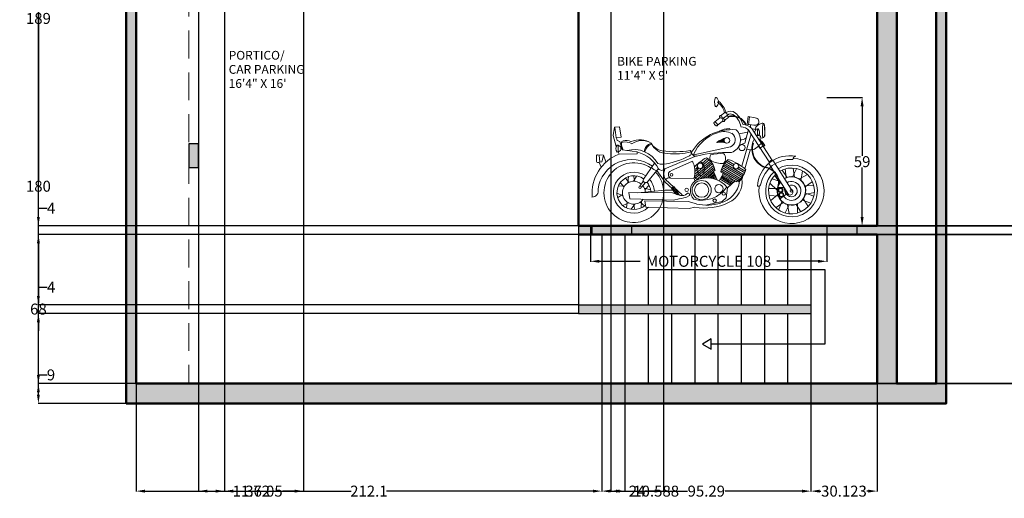
# Model space of a CAD drawing. Units: inches. Extents: x -12 to 887, y 330 to 874.
# Tile 1 of 9: x -7 to 442, y 330 to 548. Entities that reach past the tile are written whole.
import ezdxf

# ---------------------------------------------------------------- set-up
doc = ezdxf.new("R2010")
doc.units = ezdxf.units.IN
doc.header["$MEASUREMENT"] = 0
doc.linetypes.add('DASHED', pattern=[19.05, 12.7, -6.35])
for name, color, linetype, lineweight in [('A-ANNO-DIMS', 2, 'Continuous', 18), ('A-AREA-IDEN', 7, 'Continuous', 18), ('A-EQPM', 8, 'Continuous', 18), ('A-FLOR-STRS', 3, 'Continuous', 25), ('A-GLAZ', 4, 'Continuous', 25), ('A-WALL', 7, 'Continuous', 50), ('A-WALL-OVHD', 8, 'DASHED', 18), ('A-WALL-PATT', 5, 'Continuous', 13)]:
    doc.layers.add(name, color=color, linetype=linetype, lineweight=lineweight)
doc.styles.get("Standard").update_dxf_attribs({"font": 'arial.ttf'})
doc.dimstyles.get("Standard").update_dxf_attribs({"dimtxt": 5, "dimasz": 4, "dimexe": 0.18, "dimexo": 0.0625, "dimgap": 0.09, "dimtad": 0, "dimtih": 1, "dimtoh": 1, "dimdec": 1, "dimzin": 0, "dimdsep": 46, "dimlunit": 4, "dimtxsty": 'Standard', "dimcen": 0.09, "dimadec": 0, "dimazin": 0, "dimtfac": 1, "dimtdec": 1, "dimtofl": 0, "dimtmove": 0, "dimatfit": 3, "dimfxl": 1, "dimtolj": 1, "dimtzin": 0, "dimarcsym": 0})

# ---------------------------------------------------------------- blocks, each defined once
blk = doc.blocks.new('7')
at = {"color": 0}
for p, q in [((3892, 8882), (3935, 8915)), ((3832, 8822), (3885, 8862)), ((3856, 8784), (3912, 8827)), ((3881, 8881), (3905, 8892)), ((3961, 8887), (3922, 8856)), ((3930, 8837), (3971, 8866)), ((3930, 8825), (3937, 8842)), ((4161, 8796), (4172, 8876)), ((4244, 8861), (4172, 8876)), ((4175, 8791), (4186, 8872)), ((2802, 8682), (2815, 8766)), ((2864, 8771), (2815, 8766)), ((2819, 8766), (2832, 8656)), ((2864, 8771), (2882, 8664)), ((4165, 8714), (4080, 8699)), ((4174, 8741), (4138, 8602)), ((4229, 8787), (4161, 8796)), ((4183, 8727), (4385, 8415)), ((4196, 8788), (4196, 8761)), ((4414, 8434), (4208, 8753)), ((4211, 8749), (4253, 8742)), ((4267, 8749), (4267, 8680)), ((4267, 8749), (4275, 8749)), ((4273, 8784), (4268, 8793)), ((4340, 8677), (4337, 8787)), ((2833, 8569), (2802, 8682)), ((2882, 8664), (2832, 8656)), ((2842, 8629), (2834, 8656)), ((2867, 8622), (2842, 8629)), ((2892, 8535), (2867, 8622)), ((4138, 8602), (4080, 8582)), ((4203, 8697), (4107, 8368)), ((4310, 8603), (4273, 8578)), ((4276, 8680), (4276, 8680)), ((4296, 8670), (4283, 8688)), ((4290, 8644), (4296, 8670)), ((4310, 8615), (4290, 8644)), ((4315, 8619), (4303, 8607)), ((4327, 8577), (4310, 8603)), ((4342, 8579), (4315, 8619)), ((2841, 8513), (2841, 8513)), ((2850, 8582), (2843, 8582)), ((2851, 8582), (2851, 8513)), ((2861, 8492), (2852, 8513)), ((3045, 8514), (2892, 8535)), ((3046, 8515), (3046, 8495)), ((4139, 8343), (4193, 8532)), ((4290, 8552), (4273, 8578)), ((4327, 8577), (4290, 8552)), ((4342, 8579), (4326, 8571)), ((2632, 8417), (2631, 8474)), ((2641, 8484), (2702, 8482)), ((2658, 8408), (2642, 8408)), ((2658, 8482), (2665, 8410)), ((2678, 8360), (2658, 8408)), ((2660, 8410), (2687, 8415)), ((2687, 8415), (2702, 8477)), ((2702, 8482), (2727, 8413)), ((3046, 8495), (2861, 8492)), ((3222, 8401), (3109, 8238)), ((3388, 8321), (3605, 8421)), ((3800, 8406), (3627, 8261)), ((3787, 8418), (3631, 8287)), ((3763, 8446), (3702, 8395)), ((3776, 8435), (3711, 8380)), ((4021, 8371), (3947, 8415)), ((4028, 8387), (3960, 8428)), ((4385, 8415), (4382, 8396)), ((4385, 8415), (4414, 8434)), ((4414, 8434), (4422, 8429)), ((4422, 8429), (4625, 8108)), ((3260, 8345), (3149, 8210)), ((3330, 8206), (3245, 8326)), ((3660, 8360), (3631, 8336)), ((3673, 8348), (3632, 8314)), ((3808, 8393), (3636, 8249)), ((3819, 8377), (3650, 8235)), ((3826, 8360), (3684, 8241)), ((3831, 8344), (3716, 8247)), ((3825, 8304), (3762, 8250)), ((3858, 8230), (3820, 8315)), ((4070, 8221), (3897, 8323)), ((4083, 8230), (3901, 8338)), ((4096, 8242), (3907, 8355)), ((4108, 8259), (3916, 8373)), ((4118, 8270), (3923, 8386)), ((4124, 8286), (3933, 8400)), ((4137, 8302), (4064, 8346)), ((4143, 8319), (4075, 8359)), ((4382, 8396), (4583, 8080)), ((4517, 8329), (4568, 8256)), ((4557, 8250), (4547, 8343)), ((4623, 8262), (4663, 8343)), ((4644, 8258), (4628, 8350)), ((4708, 8224), (4725, 8320)), ((2876, 8201), (2910, 8159)), ((2927, 8249), (2961, 8206)), ((2957, 8263), (2950, 8200)), ((3009, 8271), (3021, 8216)), ((3038, 8269), (3009, 8216)), ((3108, 8219), (3072, 8167)), ((3130, 8203), (3087, 8156)), ((3328, 8206), (3473, 8076)), ((3333, 8233), (3501, 8079)), ((3385, 8249), (3622, 8243)), ((3622, 8243), (3631, 8223)), ((3831, 8292), (3780, 8249)), ((3836, 8280), (3797, 8247)), ((3841, 8268), (3813, 8244)), ((3847, 8254), (3830, 8240)), ((3919, 8293), (3876, 8222)), ((3989, 8176), (3886, 8237)), ((4001, 8186), (3893, 8250)), ((4010, 8195), (3900, 8261)), ((4020, 8204), (3906, 8272)), ((4029, 8213), (3912, 8282)), ((4039, 8221), (3962, 8150)), ((4077, 8211), (4064, 8218)), ((4116, 8250), (4077, 8211)), ((4116, 8250), (4113, 8263)), ((4498, 8213), (4417, 8240)), ((4442, 8275), (4493, 8199)), ((4687, 8237), (4774, 8285)), ((4750, 8159), (4824, 8213)), ((2857, 8170), (2916, 8167)), ((3402, 8097), (2961, 8101)), ((2969, 8037), (2961, 8101)), ((3329, 8126), (3051, 8100)), ((3118, 8147), (3180, 8130)), ((3165, 8176), (3123, 8130)), ((3420, 8126), (3329, 8126)), ((3416, 8154), (3396, 8137)), ((3424, 8148), (3406, 8131)), ((3431, 8137), (3412, 8121)), ((3439, 8127), (3416, 8113)), ((3447, 8115), (3424, 8102)), ((3449, 8109), (3427, 8096)), ((3962, 8149), (3947, 8047)), ((4383, 8143), (4471, 8142)), ((4393, 8197), (4468, 8127)), ((4473, 8152), (4473, 8094)), ((4534, 8152), (4473, 8152)), ((4553, 8080), (4534, 8152)), ((4742, 8173), (4839, 8169)), ((4752, 8081), (4844, 8102)), ((2840, 8096), (2899, 8068)), ((2895, 8083), (2846, 8049)), ((2942, 8005), (2935, 7947)), ((3412, 8024), (2969, 8037)), ((3075, 8003), (3118, 7966)), ((3087, 8012), (3086, 7946)), ((3123, 8017), (3564, 8012)), ((3131, 7952), (3123, 8017)), ((3402, 8097), (3484, 8072)), ((3470, 8038), (3412, 8024)), ((3564, 8012), (3646, 7987)), ((3755, 7975), (3908, 8010)), ((3947, 8047), (3908, 8010)), ((4387, 8070), (4482, 8064)), ((4474, 8083), (4402, 8021)), ((4473, 8094), (4499, 8042)), ((4514, 8008), (4480, 7924)), ((4499, 8042), (4553, 8080)), ((4554, 8080), (4581, 8082)), ((4723, 8024), (4808, 7995)), ((4731, 8041), (4781, 7960)), ((4754, 8094), (4838, 8065)), ((2959, 7996), (2899, 7971)), ((3022, 7984), (2985, 7931)), ((3006, 7983), (3022, 7929)), ((3574, 7940), (3131, 7952)), ((3631, 7954), (3574, 7940)), ((4455, 7949), (4528, 8000)), ((4547, 7895), (4587, 7976)), ((4572, 7978), (4587, 7887)), ((4661, 7981), (4706, 7906)), ((4674, 7987), (4674, 7894))]:
    blk.add_line(p, q, dxfattribs=at)
for points in [[(3849, 9066, 0.260683), (3844, 9068, 0.210261), (3839, 9065, 0.074112), (3836, 9057, 0.038164), (3832, 9041, 0.027841), (3831, 9024, 0.026604), (3832, 9007, 0.032948), (3834, 8990, 0.055713), (3838, 8981, 0.142828), (3843, 8975, 0.295184), (3847, 8975, 0.138472)], [(3914, 8827, 0.091874), (3925, 8823, 0.221617), (3930, 8824, 0.223926), (3932, 8828, 0.093027), (3930, 8839, 0.049734), (3924, 8850, 0.038285), (3915, 8863, 0.040277), (3903, 8874, 0.058568), (3894, 8880, 0.124681), (3885, 8882, 0.261773), (3881, 8879, 0.168516), (3880, 8874, 0.071525), (3884, 8862, 0.04375)]]:
    blk.add_lwpolyline(points, format="xyb", dxfattribs=at)
for points in [[(3827, 8817, 0.170081), (3825, 8813, 0.104992), (3825, 8806, 0.066813), (3828, 8799, 0.052957), (3833, 8791, 0.052957), (3840, 8785, 0.066813), (3847, 8781, 0.104992), (3853, 8780, 0.170081), (3858, 8781, 0.170081), (3860, 8785, 0.104992), (3860, 8792, 0.066813), (3857, 8799, 0.052957), (3851, 8807, 0.052957), (3844, 8814, 0.066813), (3838, 8817, 0.104992), (3831, 8818, 0.170081)], [(3687, 8412, 0.164525), (3674, 8407, 0.105794), (3661, 8390, 0.0691), (3655, 8369, 0.055299), (3653, 8342, 0.055299), (3657, 8314, 0.0691), (3666, 8294, 0.105794), (3680, 8279, 0.164525), (3693, 8275, 0.164525), (3706, 8280, 0.105794), (3718, 8296, 0.0691), (3725, 8318, 0.055299), (3727, 8345, 0.055299), (3722, 8372, 0.0691), (3714, 8393, 0.105794), (3700, 8408, 0.164525)]]:
    blk.add_lwpolyline(points, format="xyb", close=True, dxfattribs=at)
blk.add_lwpolyline([(3456, 8104), (3417, 8162), (3395, 8146), (3434, 8089)], close=True, dxfattribs=at)
for centre, radius in [((3956, 8632), 29), ((4109, 8559), 31.6), ((3684, 8374), 27.8), ((4049, 8369), 27.8), ((3394, 8282), 13.4), ((3700, 8126), 97.7), ((3075, 8156), 11.9), ((3453, 8090), 11.8), ((3547, 8129), 17.5), ((3700, 8126), 73), ((3875, 8141), 43), ((3924, 8090), 16.6), ((4501, 8126), 23.6), ((4501, 8125), 17.8), ((4509, 8079), 23.6), ((4612, 8118), 13.5), ((3832, 8019), 18.1), ((3832, 8019), 14.9), ((4509, 8078), 17.8)]:
    blk.add_circle(centre, radius, dxfattribs=at)
for centre, radius, start, end in [((3817, 9021), 55.4, 301.5348, 58.4652), ((3873, 9019), 9.82, 104.0978, 252.207), ((3767, 8879), 168, 11.2815, 51.1802), ((3715, 8844), 243, 16.6671, 49.3391), ((3947, 8966), 52.6, 257.6806, 271.9306), ((3936, 8888), 25.4, 349.901, 92.6362), ((3993, 8858), 71.6, 45.751, 128.5242), ((3994, 8851), 49.7, 61.2951, 128.7444), ((3914, 8745), 209, 14.1319, 51.6883), ((3890, 8837), 25.6, 342.4128, 100.8543), ((3997, 8888), 34.6, 175.8448, 217.5537), ((4008, 8719), 162, 25.0285, 106.0034), ((4011, 8727), 148, 25.1937, 107.8697), ((3918, 8743), 182, 8.9726, 56.7456), ((4242, 8823), 38.2, 249.4931, 86.5546), ((4336, 8702), 106, 102.6793, 157.3086), ((4317, 8786), 19.9, 1.5622, 102.6793), ((4700, 8724), 384, 167.9842, 189.8124), ((4005, 8262), 479, 84.5439, 148.5469), ((3982, 8330), 398, 107.8027, 156.6864), ((3925, 8549), 173, 61.9431, 112.2352), ((3974, 8573), 179, 88.2753, 122.4065), ((3975, 8740), 13.1, 5.9061, 67.8337), ((3965, 8639), 76.8, 290.0846, 57.4638), ((3954, 8639), 140, 290.1355, 45.6942), ((4096, 8664), 107, 36.4358, 89.1678), ((4104, 8650), 146, 44.5554, 85.2579), ((4273, 8715), 34.6, 99.9039, 275.8028), ((4239, 8714), 49.7, 317.4334, 44.5421), ((4038, 8723), 305, 351.2674, 12.4234), ((2905, 8608), 19.9, 95.9816, 177.5473), ((3031, 8603), 146, 177.5473, 208.4219), ((2926, 8491), 125, 58.4176, 107.3752), ((2932, 8523), 109, 62.7222, 105.2846), ((3070, 8426), 212, 56.195, 114.4758), ((3094, 8452), 178, 58.6083, 125.21), ((3219, 8503), 106, 108.2065, 171.3208), ((3346, 8673), 174, 203.6371, 272.1504), ((3318, 8670), 146, 207.4738, 261.8116), ((3889, 8408), 206, 73.0528, 100.6458), ((4056, 8337), 341, 109.1415, 126.3424), ((4055, 8331), 341, 111.0502, 124.5482), ((4057, 8327), 341, 112.1061, 123.1387), ((4059, 8323), 341, 112.7281, 121.53), ((4062, 8318), 341, 113.2869, 120.0065), ((4064, 8313), 341, 113.6156, 118.3049), ((4068, 8309), 341, 113.9261, 117.0275), ((4106, 8699), 61.6, 257.0918, 317.0437), ((4415, 8547), 206, 152.0409, 248.4801), ((4408, 8542), 192, 161.4337, 248.7012), ((4307, 8690), 35.4, 244.8132, 337.421), ((2878, 8547), 49.7, 135.4579, 222.5666), ((2844, 8548), 34.6, 264.1972, 80.0961), ((3014, 8265), 273, 28.4539, 105.7812), ((2968, 8195), 328, 26.8571, 76.3038), ((3226, 8493), 106, 108.2065, 168.0273), ((3431, 9401), 885, 261.4777, 279.8394), ((3426, 9194), 699, 263.9454, 283.7855), ((3564, 8504), 30.4, 293.3852, 52.3647), ((3639, 8516), 43.9, 185.4038, 280.8564), ((-29543, 159103), 154226, 282.41752, 282.55865), ((3951, 7189), 1319, 87.801, 103.311), ((4198, 8633), 97.7, 245.4669, 322.6056), ((3014, 8093), 428, 110.9827, 185.1629), ((2641, 8474), 10, 88.0251, 181.7899), ((2642, 8418), 10, 181.7899, 270), ((2992, 8089), 348, 53.5109, 172.5458), ((3011, 8100), 304, 54.9708, 43.6394), ((3198, 9180), 799, 277.8005, 298.2391), ((8228, -3327), 12658, 111.2159, 112.7855), ((3399, 8313), 233, 342.5746, 27.8143), ((3968, 8044), 466, 117.9514, 137.0146), ((3646, 8293), 192, 10.3511, 57.404), ((3845, 8455), 62.2, 151.2359, 203.559), ((3911, 8645), 248, 240.2658, 272.6625), ((3904, 7984), 513, 87.7369, 102.8433), ((4085, 8282), 192, 126.7869, 171.5108), ((3864, 8449), 77.6, 318.9005, 41.0995), ((3831, 7992), 466, 47.2214, 73.0089), ((4597, 8144), 332, 79.5967, 176.3465), ((4612, 8118), 331, 172.2424, 87.4437), ((4607, 8126), 313, 86.4681, 168.0724), ((4665, 8433), 38.7, 101.9603, 170.9773), ((3011, 8100), 209, 54.7941, 314.7174), ((3242, 8379), 53.5, 201.3616, 272.5452), ((3298, 8535), 146, 252.5701, 273.1798), ((3294, 8367), 40.4, 216.5014, 323.4986), ((3424, 8293), 108, 154.2684, 215.8165), ((3400, 8284), 38.3, 108.4812, 246.3137), ((1659, 10859), 3338, 308.5952, 310.6894), ((5726, 11101), 3338, 236.7238, 239.9594), ((3960, 8379), 192, 299.6211, 346.674), ((4327, 8203), 158, 353.693, 86.0794), ((4327, 8203), 153, 338.331, 85.2975), ((4612, 8118), 263, 131.3252, 121.2117), ((4612, 8118), 233, 132.1166, 121.0692), ((3011, 8100), 172, 54.6709, 312.9747), ((3011, 8100), 116, 49.5714, 141.177), ((3131, 8227), 24.7, 153.8384, 315.8932), ((3011, 8100), 172, 4.2846, 38.6149), ((3011, 8100), 209, 4.3358, 40.487), ((3364, 8218), 33.5, 70.6699, 154.2406), ((3708, 8122), 123, 124.8856, 225.2602), ((3778, 8379), 192, 217.8777, 230.3607), ((3755, 7982), 268, 39.0684, 116.0302), ((3830, 8242), 254, 282.4184, 354.4459), ((3876, 8213), 235, 294.264, 7.2031), ((4612, 8118), 145, 140.9316, 120.3235), ((4612, 8118), 143, 140.9316, 114.9418), ((4612, 8118), 95.7, 213.5351, 119.3096), ((2585, 8119), 64.5, 270.4315, 13.571), ((3011, 8100), 116, 141.177, 324.8838), ((3011, 8100), 116, 3.7463, 37.9624), ((3702, 8325), 302, 254.4518, 326.5201), ((4273, 8193), 28.3, 256.2637, 355.791), ((4612, 8118), 59.3, 172.2875, 117.4707), ((4597, 8104), 27.7, 238.2022, 8.1755), ((3453, 8283), 245, 273.8182, 298.0782), ((3498, 8150), 79.9, 260.2721, 309.8649), ((3561, 8080), 15.3, 299.2076, 144.0595), ((3732, 8500), 556, 259.5604, 295.6289), ((3750, 8493), 519, 258.7337, 285.941)]:
    blk.add_arc(centre, radius, start, end, dxfattribs=at)
blk = doc.blocks.new('*D36')
at = {"layer": 'A-ANNO-DIMS', "color": 0, "lineweight": -2, "transparency": 16777216}
for p, q in [((253.42, 454), (253.42, 437.75)), ((361, 454), (361, 437.75)), ((257.42, 437.93), (276.09, 437.93)), ((357, 437.93), (338.33, 437.93))]:
    blk.add_line(p, q, dxfattribs=at)
at = {"layer": 'A-ANNO-DIMS', "color": 0, "transparency": 16777216}
for points in [[(257.42, 438.6), (257.42, 437.26), (253.42, 437.93)], [(357, 438.6), (357, 437.26), (361, 437.93)]]:
    blk.add_solid(points, dxfattribs=at)
at = {"layer": 'Defpoints', "color": 0, "transparency": 16777216}
for p in [(253.42, 454.07), (361, 454.07), (361, 437.93)]:
    blk.add_point(p, dxfattribs=at)
at = {"layer": 'A-ANNO-DIMS', "color": 0, "transparency": 16777216, "insert": (307.21, 437.93), "char_height": 5, "attachment_point": 5}
blk.add_mtext('\\A1;MOTORCYCLE 108', dxfattribs=at)
blk = doc.blocks.new('*D37')
at = {"layer": 'A-ANNO-DIMS', "color": 0, "lineweight": -2, "transparency": 16777216}
for p, q in [((361.06, 512.64), (377.32, 512.64)), ((377.14, 508.64), (377.14, 486)), ((377.14, 458.07), (377.14, 480.71)), ((361.06, 454.07), (377.32, 454.07))]:
    blk.add_line(p, q, dxfattribs=at)
at = {"layer": 'A-ANNO-DIMS', "color": 0, "transparency": 16777216}
for points in [[(376.47, 508.64), (377.8, 508.64), (377.14, 512.64)], [(376.47, 458.07), (377.8, 458.07), (377.14, 454.07)]]:
    blk.add_solid(points, dxfattribs=at)
at = {"layer": 'Defpoints', "color": 0, "transparency": 16777216}
for p in [(361, 512.64), (377.14, 512.64), (361, 454.07)]:
    blk.add_point(p, dxfattribs=at)
at = {"layer": 'A-ANNO-DIMS', "color": 0, "transparency": 16777216, "insert": (377.14, 483.35), "char_height": 5, "attachment_point": 5}
blk.add_mtext('\\A1;59', dxfattribs=at)
blk = doc.blocks.new('*D50')
at = {"layer": 'A-ANNO-DIMS', "color": 0, "lineweight": -2, "transparency": 16777216}
for p, q in [((46.43, 382.1), (46.43, 332.98)), ((258.51, 382.1), (258.51, 332.98)), ((50.43, 333.16), (144.38, 333.16)), ((254.51, 333.16), (160.56, 333.16))]:
    blk.add_line(p, q, dxfattribs=at)
at = {"layer": 'A-ANNO-DIMS', "color": 0, "transparency": 16777216}
for points in [[(50.43, 333.83), (50.43, 332.49), (46.43, 333.16)], [(254.51, 333.83), (254.51, 332.49), (258.51, 333.16)]]:
    blk.add_solid(points, dxfattribs=at)
at = {"layer": 'Defpoints', "color": 0, "transparency": 16777216}
for p in [(46.43, 382.16), (258.51, 382.16), (258.51, 333.16)]:
    blk.add_point(p, dxfattribs=at)
at = {"layer": 'A-ANNO-DIMS', "color": 0, "transparency": 16777216, "insert": (152.47, 333.16), "char_height": 5, "attachment_point": 5}
blk.add_mtext('\\A1;212.1', dxfattribs=at)
blk = doc.blocks.new('*D51')
at = {"layer": 'A-ANNO-DIMS', "color": 0, "lineweight": -2, "transparency": 16777216}
for p, q in [((258.51, 382.1), (258.51, 332.98)), ((353.8, 382.1), (353.8, 332.98)), ((262.51, 333.16), (297.63, 333.16)), ((349.8, 333.16), (314.69, 333.16))]:
    blk.add_line(p, q, dxfattribs=at)
at = {"layer": 'A-ANNO-DIMS', "color": 0, "transparency": 16777216}
for points in [[(262.51, 333.83), (262.51, 332.49), (258.51, 333.16)], [(349.8, 333.83), (349.8, 332.49), (353.8, 333.16)]]:
    blk.add_solid(points, dxfattribs=at)
at = {"layer": 'Defpoints', "color": 0, "transparency": 16777216}
for p in [(258.51, 382.16), (353.8, 382.16), (353.8, 333.16)]:
    blk.add_point(p, dxfattribs=at)
at = {"layer": 'A-ANNO-DIMS', "color": 0, "transparency": 16777216, "insert": (306.16, 333.16), "char_height": 5, "attachment_point": 5}
blk.add_mtext('\\A1;95.29', dxfattribs=at)
blk = doc.blocks.new('*D52')
at = {"layer": 'A-ANNO-DIMS', "color": 0, "lineweight": -2, "transparency": 16777216}
for p, q in [((353.8, 382.1), (353.8, 332.98)), ((383.93, 382.1), (383.93, 332.98)), ((357.8, 333.16), (358.4, 333.16)), ((379.93, 333.16), (379.33, 333.16))]:
    blk.add_line(p, q, dxfattribs=at)
at = {"layer": 'A-ANNO-DIMS', "color": 0, "transparency": 16777216}
for points in [[(357.8, 333.83), (357.8, 332.49), (353.8, 333.16)], [(379.93, 333.83), (379.93, 332.49), (383.93, 333.16)]]:
    blk.add_solid(points, dxfattribs=at)
at = {"layer": 'Defpoints', "color": 0, "transparency": 16777216}
for p in [(353.8, 382.16), (383.93, 382.16), (383.93, 333.16)]:
    blk.add_point(p, dxfattribs=at)
at = {"layer": 'A-ANNO-DIMS', "color": 0, "transparency": 16777216, "insert": (368.86, 333.16), "char_height": 5, "attachment_point": 5}
blk.add_mtext('\\A1;30.123', dxfattribs=at)
blk = doc.blocks.new('*D53')
at = {"layer": 'A-ANNO-DIMS', "color": 0, "lineweight": -2, "transparency": 16777216}
for p, q in [((41.86, 830.66), (1.75, 830.66)), ((1.93, 826.66), (1.93, 604.54)), ((1.93, 377.16), (1.93, 599.28)), ((41.86, 373.16), (1.75, 373.16))]:
    blk.add_line(p, q, dxfattribs=at)
at = {"layer": 'A-ANNO-DIMS', "color": 0, "transparency": 16777216}
for points in [[(1.26, 826.66), (2.59, 826.66), (1.93, 830.66)], [(1.26, 377.16), (2.59, 377.16), (1.93, 373.16)]]:
    blk.add_solid(points, dxfattribs=at)
at = {"layer": 'Defpoints', "color": 0, "transparency": 16777216}
for p in [(1.93, 830.66), (41.93, 830.66), (41.93, 373.16)]:
    blk.add_point(p, dxfattribs=at)
at = {"layer": 'A-ANNO-DIMS', "color": 0, "transparency": 16777216, "insert": (1.93, 601.91), "char_height": 5, "attachment_point": 5}
blk.add_mtext('\\A1;457.5', dxfattribs=at)
blk = doc.blocks.new('*D54')
at = {"layer": 'A-ANNO-DIMS', "color": 0, "lineweight": -2, "transparency": 16777216}
for p, q in [((1.93, 382.16), (1.93, 386.16)), ((1.93, 386.16), (5.93, 386.16)), ((46.36, 382.16), (1.75, 382.16)), ((1.93, 377.16), (1.93, 378.16)), ((41.86, 373.16), (1.75, 373.16))]:
    blk.add_line(p, q, dxfattribs=at)
at = {"layer": 'A-ANNO-DIMS', "color": 0, "transparency": 16777216}
for points in [[(1.26, 378.16), (2.59, 378.16), (1.93, 382.16)], [(1.26, 377.16), (2.59, 377.16), (1.93, 373.16)]]:
    blk.add_solid(points, dxfattribs=at)
at = {"layer": 'Defpoints', "color": 0, "transparency": 16777216}
for p in [(1.93, 382.16), (46.43, 382.16), (41.93, 373.16)]:
    blk.add_point(p, dxfattribs=at)
at = {"layer": 'A-ANNO-DIMS', "color": 0, "transparency": 16777216, "insert": (7.66, 386.16), "char_height": 5, "attachment_point": 5}
blk.add_mtext('\\A1;9', dxfattribs=at)
blk = doc.blocks.new('*D55')
at = {"layer": 'A-ANNO-DIMS', "color": 0, "lineweight": -2, "transparency": 16777216}
for p, q in [((70.36, 562.16), (1.75, 562.16)), ((1.93, 558.16), (1.93, 474.8)), ((1.93, 386.16), (1.93, 469.52)), ((70.36, 382.16), (1.75, 382.16))]:
    blk.add_line(p, q, dxfattribs=at)
at = {"layer": 'A-ANNO-DIMS', "color": 0, "transparency": 16777216}
for points in [[(1.26, 558.16), (2.59, 558.16), (1.93, 562.16)], [(1.26, 386.16), (2.59, 386.16), (1.93, 382.16)]]:
    blk.add_solid(points, dxfattribs=at)
at = {"layer": 'Defpoints', "color": 0, "transparency": 16777216}
for p in [(1.93, 562.16), (70.43, 562.16), (70.43, 382.16)]:
    blk.add_point(p, dxfattribs=at)
at = {"layer": 'A-ANNO-DIMS', "color": 0, "transparency": 16777216, "insert": (1.93, 472.16), "char_height": 5, "attachment_point": 5}
blk.add_mtext('\\A1;180', dxfattribs=at)
blk = doc.blocks.new('*D60')
at = {"layer": 'A-ANNO-DIMS', "color": 0, "lineweight": -2, "transparency": 16777216}
for p, q in [((383.99, 450.16), (873.75, 450.16)), ((873.57, 446.16), (873.57, 418.8)), ((873.57, 386.16), (873.57, 413.52)), ((383.99, 382.16), (873.75, 382.16))]:
    blk.add_line(p, q, dxfattribs=at)
at = {"layer": 'A-ANNO-DIMS', "color": 0, "transparency": 16777216}
for points in [[(872.9, 446.16), (874.24, 446.16), (873.57, 450.16)], [(872.9, 386.16), (874.24, 386.16), (873.57, 382.16)]]:
    blk.add_solid(points, dxfattribs=at)
at = {"layer": 'Defpoints', "color": 0, "transparency": 16777216}
for p in [(383.93, 450.16), (873.57, 450.16), (383.93, 382.16)]:
    blk.add_point(p, dxfattribs=at)
at = {"layer": 'A-ANNO-DIMS', "color": 0, "transparency": 16777216, "insert": (873.57, 416.16), "char_height": 5, "attachment_point": 5}
blk.add_mtext('\\A1;68', dxfattribs=at)
blk = doc.blocks.new('*D61')
at = {"layer": 'A-ANNO-DIMS', "color": 0, "lineweight": -2, "transparency": 16777216}
for p, q in [((873.57, 458.16), (873.57, 462.16)), ((873.57, 462.16), (877.57, 462.16)), ((383.99, 454.16), (873.75, 454.16)), ((383.99, 450.16), (873.75, 450.16)), ((873.57, 446.16), (873.57, 442.16))]:
    blk.add_line(p, q, dxfattribs=at)
at = {"layer": 'A-ANNO-DIMS', "color": 0, "transparency": 16777216}
for points in [[(872.9, 458.16), (874.24, 458.16), (873.57, 454.16)], [(872.9, 446.16), (874.24, 446.16), (873.57, 450.16)]]:
    blk.add_solid(points, dxfattribs=at)
at = {"layer": 'Defpoints', "color": 0, "transparency": 16777216}
for p in [(383.93, 454.16), (873.57, 454.16), (383.93, 450.16)]:
    blk.add_point(p, dxfattribs=at)
at = {"layer": 'A-ANNO-DIMS', "color": 0, "transparency": 16777216, "insert": (879.39, 462.16), "char_height": 5, "attachment_point": 5}
blk.add_mtext('\\A1;4', dxfattribs=at)
blk = doc.blocks.new('*D62')
at = {"layer": 'A-ANNO-DIMS', "color": 0, "lineweight": -2, "transparency": 16777216}
for p, q in [((383.99, 562.16), (873.75, 562.16)), ((873.57, 558.16), (873.57, 510.8)), ((873.57, 458.16), (873.57, 505.52)), ((383.99, 454.16), (873.75, 454.16))]:
    blk.add_line(p, q, dxfattribs=at)
at = {"layer": 'A-ANNO-DIMS', "color": 0, "transparency": 16777216}
for points in [[(872.9, 558.16), (874.24, 558.16), (873.57, 562.16)], [(872.9, 458.16), (874.24, 458.16), (873.57, 454.16)]]:
    blk.add_solid(points, dxfattribs=at)
at = {"layer": 'Defpoints', "color": 0, "transparency": 16777216}
for p in [(383.93, 562.16), (873.57, 562.16), (383.93, 454.16)]:
    blk.add_point(p, dxfattribs=at)
at = {"layer": 'A-ANNO-DIMS', "color": 0, "transparency": 16777216, "insert": (873.57, 508.16), "char_height": 5, "attachment_point": 5}
blk.add_mtext('\\A1;108', dxfattribs=at)
blk = doc.blocks.new('*D74')
at = {"layer": 'A-ANNO-DIMS', "color": 0, "lineweight": -2, "transparency": 16777216}
for p, q in [((1.93, 422.16), (1.93, 426.16)), ((1.93, 426.16), (5.93, 426.16)), ((247.86, 418.16), (1.75, 418.16)), ((247.86, 414.16), (1.75, 414.16)), ((1.93, 410.16), (1.93, 406.16))]:
    blk.add_line(p, q, dxfattribs=at)
at = {"layer": 'A-ANNO-DIMS', "color": 0, "transparency": 16777216}
for points in [[(1.26, 422.16), (2.59, 422.16), (1.93, 418.16)], [(1.26, 410.16), (2.59, 410.16), (1.93, 414.16)]]:
    blk.add_solid(points, dxfattribs=at)
at = {"layer": 'Defpoints', "color": 0, "transparency": 16777216}
for p in [(1.93, 418.16), (247.93, 418.16), (247.93, 414.16)]:
    blk.add_point(p, dxfattribs=at)
at = {"layer": 'A-ANNO-DIMS', "color": 0, "transparency": 16777216, "insert": (7.75, 426.16), "char_height": 5, "attachment_point": 5}
blk.add_mtext('\\A1;4', dxfattribs=at)
blk = doc.blocks.new('*D75')
at = {"layer": 'A-ANNO-DIMS', "color": 0, "lineweight": -2, "transparency": 16777216}
for p, q in [((258.51, 418.1), (258.51, 332.98)), ((269.1, 418.1), (269.1, 332.98)), ((262.51, 333.16), (265.1, 333.16)), ((269.1, 333.16), (273.1, 333.16))]:
    blk.add_line(p, q, dxfattribs=at)
at = {"layer": 'A-ANNO-DIMS', "color": 0, "transparency": 16777216}
for points in [[(262.51, 333.83), (262.51, 332.49), (258.51, 333.16)], [(265.1, 333.83), (265.1, 332.49), (269.1, 333.16)]]:
    blk.add_solid(points, dxfattribs=at)
at = {"layer": 'Defpoints', "color": 0, "transparency": 16777216}
for p in [(258.51, 418.16), (269.1, 418.16), (269.1, 333.16)]:
    blk.add_point(p, dxfattribs=at)
at = {"layer": 'A-ANNO-DIMS', "color": 0, "transparency": 16777216, "insert": (283.34, 333.16), "char_height": 5, "attachment_point": 5}
blk.add_mtext('\\A1;10.588', dxfattribs=at)
blk = doc.blocks.new('*D76')
at = {"layer": 'A-ANNO-DIMS', "color": 0, "lineweight": -2, "transparency": 16777216}
for p, q in [((74.93, 566.6), (74.93, 332.98)), ((86.65, 566.6), (86.65, 332.98)), ((78.93, 333.16), (82.65, 333.16)), ((86.65, 333.16), (90.65, 333.16))]:
    blk.add_line(p, q, dxfattribs=at)
at = {"layer": 'A-ANNO-DIMS', "color": 0, "transparency": 16777216}
for points in [[(78.93, 333.83), (78.93, 332.49), (74.93, 333.16)], [(82.65, 333.83), (82.65, 332.49), (86.65, 333.16)]]:
    blk.add_solid(points, dxfattribs=at)
at = {"layer": 'Defpoints', "color": 0, "transparency": 16777216}
for p in [(74.93, 566.66), (86.65, 566.66), (86.65, 333.16)]:
    blk.add_point(p, dxfattribs=at)
at = {"layer": 'A-ANNO-DIMS', "color": 0, "transparency": 16777216, "insert": (98.91, 333.16), "char_height": 5, "attachment_point": 5}
blk.add_mtext('\\A1;11.72', dxfattribs=at)
blk = doc.blocks.new('*D77')
at = {"layer": 'A-ANNO-DIMS', "color": 0, "lineweight": -2, "transparency": 16777216}
for p, q in [((86.65, 566.6), (86.65, 332.98)), ((122.7, 566.6), (122.7, 332.98)), ((90.65, 333.16), (96.13, 333.16)), ((118.7, 333.16), (113.22, 333.16))]:
    blk.add_line(p, q, dxfattribs=at)
at = {"layer": 'A-ANNO-DIMS', "color": 0, "transparency": 16777216}
for points in [[(90.65, 333.83), (90.65, 332.49), (86.65, 333.16)], [(118.7, 333.83), (118.7, 332.49), (122.7, 333.16)]]:
    blk.add_solid(points, dxfattribs=at)
at = {"layer": 'Defpoints', "color": 0, "transparency": 16777216}
for p in [(86.65, 566.66), (122.7, 566.66), (122.7, 333.16)]:
    blk.add_point(p, dxfattribs=at)
at = {"layer": 'A-ANNO-DIMS', "color": 0, "transparency": 16777216, "insert": (104.67, 333.16), "char_height": 5, "attachment_point": 5}
blk.add_mtext('\\A1;36.05', dxfattribs=at)
blk = doc.blocks.new('*D80')
at = {"layer": 'A-ANNO-DIMS', "color": 0, "lineweight": -2, "transparency": 16777216}
for p, q in [((262.63, 566.6), (262.63, 332.98)), ((286.63, 566.6), (286.63, 332.98)), ((266.63, 333.16), (270.92, 333.16)), ((282.63, 333.16), (278.33, 333.16))]:
    blk.add_line(p, q, dxfattribs=at)
at = {"layer": 'A-ANNO-DIMS', "color": 0, "transparency": 16777216}
for points in [[(266.63, 333.83), (266.63, 332.49), (262.63, 333.16)], [(282.63, 333.83), (282.63, 332.49), (286.63, 333.16)]]:
    blk.add_solid(points, dxfattribs=at)
at = {"layer": 'Defpoints', "color": 0, "transparency": 16777216}
for p in [(262.63, 566.66), (286.63, 566.66), (286.63, 333.16)]:
    blk.add_point(p, dxfattribs=at)
at = {"layer": 'A-ANNO-DIMS', "color": 0, "transparency": 16777216, "insert": (274.63, 333.16), "char_height": 5, "attachment_point": 5}
blk.add_mtext('\\A1;24', dxfattribs=at)
blk = doc.blocks.new('*D99')
at = {"layer": 'A-ANNO-DIMS', "color": 0, "lineweight": -2, "transparency": 16777216}
for p, q in [((493.01, 450.16), (1.75, 450.16)), ((1.93, 446.16), (1.93, 418.8)), ((1.93, 386.16), (1.93, 413.52)), ((493.01, 382.16), (1.75, 382.16))]:
    blk.add_line(p, q, dxfattribs=at)
at = {"layer": 'A-ANNO-DIMS', "color": 0, "transparency": 16777216}
for points in [[(1.26, 446.16), (2.59, 446.16), (1.93, 450.16)], [(1.26, 386.16), (2.59, 386.16), (1.93, 382.16)]]:
    blk.add_solid(points, dxfattribs=at)
at = {"layer": 'Defpoints', "color": 0, "transparency": 16777216}
for p in [(1.93, 450.16), (493.07, 450.16), (493.07, 382.16)]:
    blk.add_point(p, dxfattribs=at)
at = {"layer": 'A-ANNO-DIMS', "color": 0, "transparency": 16777216, "insert": (1.93, 416.16), "char_height": 5, "attachment_point": 5}
blk.add_mtext('\\A1;68', dxfattribs=at)
blk = doc.blocks.new('*D100')
at = {"layer": 'A-ANNO-DIMS', "color": 0, "lineweight": -2, "transparency": 16777216}
for p, q in [((1.93, 458.16), (1.93, 462.16)), ((1.93, 462.16), (5.93, 462.16)), ((493.01, 454.16), (1.75, 454.16)), ((493.01, 450.16), (1.75, 450.16)), ((1.93, 446.16), (1.93, 442.16))]:
    blk.add_line(p, q, dxfattribs=at)
at = {"layer": 'A-ANNO-DIMS', "color": 0, "transparency": 16777216}
for points in [[(1.26, 458.16), (2.59, 458.16), (1.93, 454.16)], [(1.26, 446.16), (2.59, 446.16), (1.93, 450.16)]]:
    blk.add_solid(points, dxfattribs=at)
at = {"layer": 'Defpoints', "color": 0, "transparency": 16777216}
for p in [(1.93, 454.16), (493.07, 454.16), (493.07, 450.16)]:
    blk.add_point(p, dxfattribs=at)
at = {"layer": 'A-ANNO-DIMS', "color": 0, "transparency": 16777216, "insert": (7.75, 462.16), "char_height": 5, "attachment_point": 5}
blk.add_mtext('\\A1;4', dxfattribs=at)
blk = doc.blocks.new('*D101')
at = {"layer": 'A-ANNO-DIMS', "color": 0, "lineweight": -2, "transparency": 16777216}
for p, q in [((493.01, 643.16), (1.75, 643.16)), ((1.93, 639.16), (1.93, 551.3)), ((1.93, 458.16), (1.93, 546.02)), ((493.01, 454.16), (1.75, 454.16))]:
    blk.add_line(p, q, dxfattribs=at)
at = {"layer": 'A-ANNO-DIMS', "color": 0, "transparency": 16777216}
for points in [[(1.26, 639.16), (2.59, 639.16), (1.93, 643.16)], [(1.26, 458.16), (2.59, 458.16), (1.93, 454.16)]]:
    blk.add_solid(points, dxfattribs=at)
at = {"layer": 'Defpoints', "color": 0, "transparency": 16777216}
for p in [(1.93, 643.16), (493.07, 643.16), (493.07, 454.16)]:
    blk.add_point(p, dxfattribs=at)
at = {"layer": 'A-ANNO-DIMS', "color": 0, "transparency": 16777216, "insert": (1.93, 548.66), "char_height": 5, "attachment_point": 5}
blk.add_mtext('\\A1;189', dxfattribs=at)

msp = doc.modelspace()

# ---------------------------------------------------------------- hatches: boundary and pattern name
at = {"layer": 'A-WALL-PATT'}
h = msp.add_hatch(color=256, dxfattribs=at)
h.dxf.hatch_style = 1
h.paths.add_polyline_path([(253.4263, 830.6611), (94.575, 830.6611), (94.575, 821.6611), (198.9263, 821.6611), (198.9263, 783.3094), (203.4263, 783.3094), (203.4263, 821.6611), (253.4263, 821.6611)], flags=17)
h.paths.add_polyline_path([(415.4263, 830.6611), (392.9263, 830.6611), (392.9263, 821.6611), (410.9263, 821.6611), (410.9263, 701.6611), (410.9263, 382.1611), (392.9263, 382.1611), (392.9263, 450.1611), (383.9263, 450.1611), (383.9263, 382.1611), (253.4263, 382.1611), (46.4263, 382.1611), (46.4263, 821.6611), (67.3199, 821.6611), (67.3199, 830.6611), (41.9263, 830.6611), (41.9263, 373.1611), (253.4263, 373.1611), (415.4263, 373.1611)])
h.paths.add_polyline_path([(364.023, 830.6611), (288.8031, 830.6611), (288.8031, 821.6611), (364.023, 821.6611)], flags=17)
h.paths.add_polyline_path([(257.9263, 821.6611), (253.4263, 821.6611), (253.4263, 749.6611), (203.4263, 749.6611), (203.4263, 759.3094), (198.9263, 759.3094), (198.9263, 745.1611), (253.4263, 745.1611), (253.4263, 735.8547), (257.9263, 735.8547)], flags=17)
h.paths.add_polyline_path([(257.9263, 653.338), (257.0311, 653.338), (253.4263, 653.338), (253.4263, 579.1607), (257.9263, 579.1607)], flags=17)
h.paths.add_polyline_path([(323.9263, 685.1611), (328.2749, 685.1611), (328.2749, 689.6611), (257.9263, 689.6611), (257.9263, 685.1611), (319.9263, 685.1611), (319.9263, 631.1611), (257.9263, 631.1611), (257.9263, 626.6611), (319.9263, 626.6611), (319.9263, 566.6611), (286.6409, 566.6611, -0.00931598), (286.6576, 565.7658), (286.6576, 562.1611), (383.9263, 562.1611), (383.9263, 566.6611), (323.9263, 566.6611)], flags=17)
h.paths.add_polyline_path([(142.5107, 566.6611), (135.5357, 566.6611), (135.5357, 562.1611), (142.5107, 562.1611)], flags=17)
h.paths.add_polyline_path([(253.4263, 566.6611), (229.0035, 566.6611), (229.0035, 562.1611), (253.4263, 562.1611)], flags=17)
h.paths.add_polyline_path([(262.6261, 566.6611), (257.9263, 566.6611), (257.9263, 562.1611), (262.6261, 562.1611)], flags=17)
h.paths.add_polyline_path([(392.9263, 553.5254), (383.9263, 553.5254), (383.9263, 454.1611), (392.9263, 454.1611)], flags=17)
h.paths.add_polyline_path([(353.8031, 418.1611), (247.9263, 418.1611), (247.9263, 414.1611), (353.8031, 414.1611)], flags=17)
h.paths.add_polyline_path([(374.959, 454.1611), (272.0195, 454.1611), (272.0195, 450.1611), (374.959, 450.1611)], flags=17)
h.paths.add_polyline_path([(254.2006, 454.1611), (247.9263, 454.1611), (247.9263, 450.1611), (254.2006, 450.1611)], flags=17)
h = msp.add_hatch(color=256, dxfattribs=at)
h.dxf.hatch_style = 1
h.paths.add_polyline_path([(94.575, 830.6611), (67.3199, 830.6611), (67.3199, 821.6611), (70.4263, 821.6611), (79.4263, 821.6611), (94.575, 821.6611)])
h.paths.add_polyline_path([(288.8031, 830.6611), (257.9263, 830.6611), (253.4263, 830.6611), (253.4263, 821.6611), (288.8031, 821.6611)])
h.paths.add_polyline_path([(74.9263, 696.9265), (70.4263, 696.9265), (70.4263, 678.4656), (74.9263, 678.4656)])
h.paths.add_polyline_path([(74.9263, 584.8756), (70.4263, 584.8756), (70.4263, 562.1611), (74.9263, 562.1611)])
h.paths.add_polyline_path([(135.5357, 566.6611), (122.6994, 566.6611), (122.6994, 562.1611), (135.5357, 562.1611)])
h.paths.add_polyline_path([(257.9263, 579.1607), (253.4263, 579.1607), (253.4263, 562.1611), (257.9263, 562.1611)])
h.paths.add_polyline_path([(272.0195, 454.1611), (254.2006, 454.1611), (254.2006, 450.1611), (272.0195, 450.1611)])
h.paths.add_polyline_path([(392.9263, 454.1611), (374.959, 454.1611), (374.959, 450.1611), (383.9263, 450.1611), (392.9263, 450.1611)])
h.paths.add_polyline_path([(493.0683, 466.4171), (488.5683, 466.4171), (488.5683, 450.1611), (493.0683, 450.1611)])
h.paths.add_polyline_path([(568.6302, 454.1611), (555.938, 454.1611), (555.938, 450.1611), (568.6302, 450.1611)])
h.paths.add_polyline_path([(493.0683, 594.9471), (488.5683, 594.9471), (488.5683, 569.5862), (493.0683, 569.5862)])
h.paths.add_polyline_path([(690.1615, 454.1611), (672.3426, 454.1611), (672.3426, 450.1611), (690.1615, 450.1611)])
h.paths.add_polyline_path([(811.0683, 454.1611), (793.101, 454.1611), (793.101, 450.1611), (802.0683, 450.1611), (811.0683, 450.1611)])
h.paths.add_polyline_path([(811.0683, 578.3606), (802.0683, 578.3606), (802.0683, 566.6611), (802.0683, 553.5254), (811.0683, 553.5254)])
h.paths.add_polyline_path([(811.0683, 701.6611), (802.0683, 701.6611), (802.0683, 689.9616), (802.0683, 676.8259), (811.0683, 676.8259)])
h.paths.add_polyline_path([(811.0683, 830.6611), (782.165, 830.6611), (782.165, 821.6611), (802.0683, 821.6611), (811.0683, 821.6611)])
h.paths.add_polyline_path([(706.9451, 830.6611), (671.5683, 830.6611), (671.5683, 821.6611), (706.9451, 821.6611)])
h.paths.add_polyline_path([(512.717, 830.6611), (485.4619, 830.6611), (485.4619, 821.6611), (488.5683, 821.6611), (512.717, 821.6611)])
h.paths.add_polyline_path([(392.9263, 697.8668), (383.9263, 697.8668), (383.9263, 689.6611), (383.9263, 676.5034), (392.9263, 676.5034)])
h.paths.add_polyline_path([(392.9263, 830.6611), (364.023, 830.6611), (364.023, 821.7357), (392.9263, 821.7357)])
h.paths.add_polyline_path([(392.9263, 619.0434), (383.9263, 619.0434), (383.9263, 588.7499), (392.9263, 588.7499)])
h.paths.add_polyline_path([(392.9263, 578.3606), (383.9263, 578.3606), (383.9263, 566.6611), (383.9263, 553.5254), (392.9263, 553.5254)])
h.paths.add_polyline_path([(257.9263, 699.8547), (253.4263, 699.8547), (253.4263, 697.1611), (253.4263, 677.338), (257.9263, 677.338)])
h.paths.add_polyline_path([(493.0683, 714.3785), (488.5683, 714.3785), (488.5683, 689.6611), (493.0683, 689.6611)])
h.paths.add_polyline_path([(74.9263, 491.4191), (70.4263, 491.4191), (70.4263, 480.7097), (74.9263, 480.7097)])

# ---------------------------------------------------------------- linework, layer by layer
at = {"layer": 'A-FLOR-STRS'}
for p, q in [((247.9263, 454.1611), (247.9263, 414.1611)), ((258.514, 450.1611), (258.514, 418.1611)), ((269.1017, 450.1611), (269.1017, 418.1611)), ((279.6894, 450.1611), (279.6894, 418.1611)), ((290.277, 450.1611), (290.277, 418.1611)), ((300.8647, 450.1611), (300.8647, 418.1611)), ((311.4524, 450.1611), (311.4524, 418.1611)), ((322.04, 450.1611), (322.04, 418.1611)), ((332.6277, 450.1611), (332.6277, 418.1611)), ((343.2154, 450.1611), (343.2154, 418.1611)), ((279.6894, 434.1611), (360.1054, 434.1611)), ((360.1054, 434.1611), (360.1054, 400.1611)), ((247.9263, 418.1611), (353.8031, 418.1611)), ((247.9263, 414.1611), (353.8031, 414.1611)), ((258.514, 414.1611), (258.514, 382.1611)), ((269.1017, 414.1611), (269.1017, 382.1611)), ((279.6894, 414.1611), (279.6894, 382.1611)), ((290.277, 414.1611), (290.277, 382.1611)), ((300.8647, 414.1611), (300.8647, 382.1611)), ((311.4524, 414.1611), (311.4524, 382.1611)), ((322.04, 414.1611), (322.04, 382.1611)), ((332.6277, 414.1611), (332.6277, 382.1611)), ((343.2154, 414.1611), (343.2154, 382.1611)), ((360.1054, 400.1611), (308.3988, 400.1611))]:
    msp.add_line(p, q, dxfattribs=at)
msp.add_lwpolyline([(353.8031, 450.1611), (353.8031, 418.1611), (353.8031, 382.1611)], dxfattribs=at)
msp.add_lwpolyline([(308.3988, 402.5244), (304.4077, 400.1611), (308.3988, 397.8475), (308.3988, 400.1611)], close=True, dxfattribs=at)
at = {"layer": 'A-GLAZ'}
for points in [[(70.4263, 480.7097), (74.9263, 480.7097), (74.9263, 491.4191), (70.4263, 491.4191)], [(254.2006, 454.1611), (272.0195, 454.1611), (272.0195, 450.1611), (254.2006, 450.1611)], [(374.959, 454.1611), (392.9263, 454.1611), (392.9263, 450.1611), (374.959, 450.1611)]]:
    msp.add_lwpolyline(points, close=True, dxfattribs=at)
at = {"layer": 'A-WALL'}
for p, q in [((247.9263, 562.1611), (247.9263, 454.1611)), ((383.9263, 562.1611), (383.9263, 454.1611)), ((247.9263, 454.1611), (383.9263, 454.1611))]:
    msp.add_line(p, q, dxfattribs=at)
for points in [[(41.9263, 830.6611), (253.4263, 830.6611), (257.9263, 830.6611), (415.4263, 830.6611), (415.4263, 373.1611), (253.4263, 373.1611), (41.9263, 373.1611)], [(410.9263, 821.6611), (392.9263, 821.6611), (392.9263, 382.1611), (410.9263, 382.1611), (410.9263, 701.6611)]]:
    msp.add_lwpolyline(points, close=True, dxfattribs=at)
msp.add_lwpolyline([(247.9263, 450.1611), (383.9263, 450.1611), (383.9263, 382.1611), (253.4263, 382.1611), (46.4263, 382.1611), (46.4263, 821.6611), (70.4263, 821.6611), (79.4263, 821.6611), (198.9263, 821.6611), (198.9263, 745.1611)], dxfattribs=at)
at = {"layer": 'A-WALL-OVHD'}
msp.add_line((70.4263, 562.1611), (70.4263, 382.1611), dxfattribs=at)

# ---------------------------------------------------------------- block references
at = {"layer": 'A-EQPM', "xscale": 0.0448456893790852, "yscale": 0.0448456893790852, "zscale": 0.0448456893790852}
msp.add_blockref('7', (138.1334, 105.9608), dxfattribs=at)

# ---------------------------------------------------------------- texts
at = {"layer": 'A-AREA-IDEN'}
for s, p in [('PORTICO/', (88.6026, 529.8514)), ('BIKE PARKING', (265.5222, 527.1211)), ('CAR PARKING', (88.6026, 523.4257)), ('11\'4" X 9\'', (265.5222, 520.6955)), ('16\'4" X 16\'', (88.6026, 517.0001))]:
    msp.add_text(s, height=4, dxfattribs=at).set_placement(p)

# ---------------------------------------------------------------- dimensions: what is measured, and where the dimension line sits
at = {"layer": 'A-ANNO-DIMS'}
for base, p1, p2, override, picture, middle in [((1.9263, 830.6611), (41.9263, 373.1611), (41.9263, 830.6611), {"dimdec": 1, "dimlfac": 1, "dimrnd": 0, "dimzin": 0, "dimdsep": 46, "dimlunit": 2}, '*D53', (1.9263, 601.9111)), ((1.9263, 643.1611), (493.0683, 454.1611), (493.0683, 643.1611), {"dimdec": 0, "dimlfac": 1, "dimrnd": 0, "dimzin": 0, "dimdsep": 46, "dimlunit": 2}, '*D101', (1.9263, 548.6611)), ((1.9263, 562.1611), (70.4263, 382.1611), (70.4263, 562.1611), {"dimdec": 0, "dimlfac": 1, "dimrnd": 0, "dimzin": 0, "dimdsep": 46, "dimlunit": 2}, '*D55', (1.9263, 472.1611)), ((873.5683, 562.1611), (383.9263, 454.1611), (383.9263, 562.1611), {"dimdec": 0, "dimlfac": 1, "dimrnd": 0, "dimzin": 0, "dimdsep": 46, "dimlunit": 2}, '*D62', (873.5683, 508.1611)), ((377.1375, 512.6428), (361.0002, 454.0662), (361.0002, 512.6428), {"dimdec": 0, "dimrnd": 0, "dimzin": 0, "dimlunit": 2}, '*D37', (377.1375, 483.3545)), ((1.9263, 454.1611), (493.0683, 450.1611), (493.0683, 454.1611), {"dimdec": 0, "dimlfac": 1, "dimrnd": 0, "dimzin": 0, "dimdsep": 46, "dimlunit": 2}, '*D100', (7.7455, 462.1611)), ((873.5683, 454.1611), (383.9263, 450.1611), (383.9263, 454.1611), {"dimdec": 0, "dimlfac": 1, "dimrnd": 0, "dimzin": 0, "dimdsep": 46, "dimlunit": 2}, '*D61', (879.3875, 462.1611)), ((1.9263, 450.1611), (493.0683, 382.1611), (493.0683, 450.1611), {"dimdec": 0, "dimlfac": 1, "dimrnd": 0, "dimzin": 0, "dimdsep": 46, "dimlunit": 2}, '*D99', (1.9263, 416.1611)), ((873.5683, 450.1611), (383.9263, 382.1611), (383.9263, 450.1611), {"dimdec": 0, "dimlfac": 1, "dimrnd": 0, "dimzin": 0, "dimdsep": 46, "dimlunit": 2}, '*D60', (873.5683, 416.1611)), ((1.9263, 418.1611), (247.9263, 414.1611), (247.9263, 418.1611), {"dimdec": 0, "dimlfac": 1, "dimrnd": 0, "dimzin": 0, "dimdsep": 46, "dimlunit": 2}, '*D74', (7.7455, 426.1611)), ((1.9263, 382.1611), (41.9263, 373.1611), (46.4263, 382.1611), {"dimdec": 0, "dimlfac": 1, "dimrnd": 0, "dimzin": 0, "dimdsep": 46, "dimlunit": 2}, '*D54', (7.6603, 386.1611))]:
    dim = msp.add_linear_dim(base=base, p1=p1, p2=p2, angle=90, dimstyle='Standard', override=override, dxfattribs=at)
    dim.commit()
    dim.dimension.update_dxf_attribs({"geometry": picture, "text_midpoint": middle})
for base, p1, p2, override, picture, middle in [((86.6469, 333.1611), (74.9263, 566.6611), (86.6469, 566.6611), {"dimdec": 2, "dimlfac": 1, "dimrnd": 0, "dimzin": 0, "dimdsep": 46, "dimlunit": 2}, '*D76', (98.9122, 333.1611)), ((122.6994, 333.1611), (86.6469, 566.6611), (122.6994, 566.6611), {"dimdec": 2, "dimlfac": 1, "dimrnd": 0, "dimzin": 0, "dimdsep": 46, "dimlunit": 2}, '*D77', (104.6732, 333.1611)), ((286.6261, 333.1611), (262.6261, 566.6611), (286.6261, 566.6611), {"dimdec": 0, "dimlfac": 1, "dimrnd": 0, "dimzin": 0, "dimdsep": 46, "dimlunit": 2}, '*D80', (274.6261, 333.1611)), ((269.1017, 333.1611), (258.514, 418.1611), (269.1017, 418.1611), {"dimdec": 3, "dimlfac": 1, "dimrnd": 0, "dimzin": 0, "dimdsep": 46, "dimlunit": 2}, '*D75', (283.34, 333.1611)), ((258.514, 333.1611), (46.4263, 382.1611), (258.514, 382.1611), {"dimdec": 1, "dimlfac": 1, "dimrnd": 0, "dimzin": 0, "dimdsep": 46, "dimlunit": 2}, '*D50', (152.4702, 333.1611)), ((353.8031, 333.1611), (258.514, 382.1611), (353.8031, 382.1611), {"dimdec": 2, "dimlfac": 1, "dimrnd": 0, "dimzin": 0, "dimdsep": 46, "dimlunit": 2}, '*D51', (306.1585, 333.1611)), ((383.9263, 333.1611), (353.8031, 382.1611), (383.9263, 382.1611), {"dimdec": 3, "dimlfac": 1, "dimrnd": 0, "dimzin": 0, "dimdsep": 46, "dimlunit": 2}, '*D52', (368.8647, 333.1611))]:
    dim = msp.add_linear_dim(base=base, p1=p1, p2=p2, dimstyle='Standard', override=override, dxfattribs=at)
    dim.commit()
    dim.dimension.update_dxf_attribs({"geometry": picture, "text_midpoint": middle})
dim = msp.add_linear_dim(base=(361.0002, 437.9288), p1=(253.418, 454.0662), p2=(361.0002, 454.0662), text='MOTORCYCLE <>', dimstyle='Standard', override={"dimdec": 0, "dimrnd": 0, "dimzin": 0, "dimlunit": 2}, dxfattribs=at)
dim.commit()
dim.dimension.update_dxf_attribs({"geometry": '*D36', "text_midpoint": (307.2091, 437.9288)})

doc.saveas('drawing.dxf')
